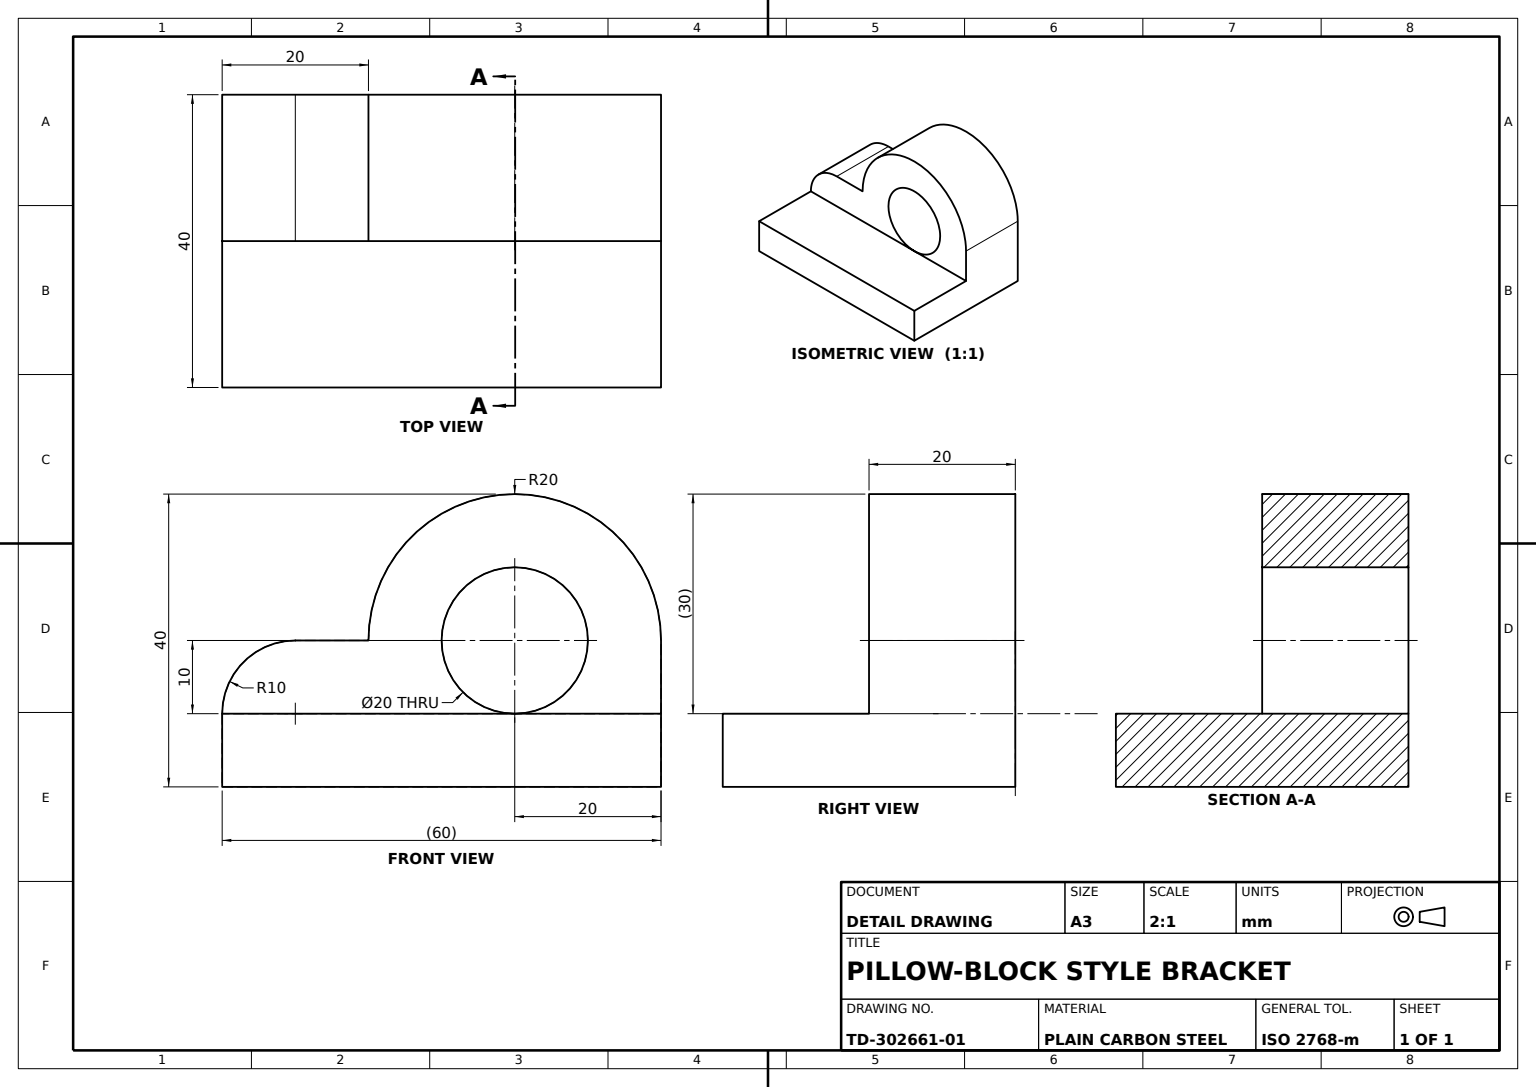
SolidWorks part; units mm, degrees
material "Plain Carbon Steel"
ref_plane "Front Plane" through (0, 0, 0) normal (0, 0, 1) x (1, 0, 0)
ref_plane "Top Plane" through (0, 0, 0) normal (0, 1, 0) x (1, 0, 0)
ref_plane "Right Plane" through (0, 0, 0) normal (1, 0, 0) x (0, 0, -1)
sketch "Base Plate Sketch" plane through (0, 0, 0) normal (0, 1, 0) x (1, 0, 0)
  line L1 (-30, -20) -> (30, -20)
  line L2 (-30, -20) -> (-30, 20)
  line L3 (-30, 20) -> (30, 20)
  line L4 (30, -20) -> (30, 20)
  line L5 (-30, -20) -> (30, 20) construction
  line L6 (-30, 20) -> (30, -20) construction
  point P0 (0, 0)
  dimension "D1" = 60
  dimension "D2" = 40
extrude "Base Plate 60x40x10" add sketch "Base Plate Sketch" along normal mid plane 10
sketch "Upright Lug Sketch" plane through (0, 5, 0) normal (0, 1, 0) x (1, 0, 0)
  line L0 (30, -20) -> (30, 20) construction
  line L1 (-30, 20) -> (30, 20)
  line L2 (-30, 20) -> (-30, 0)
  line L3 (-30, 0) -> (30, 0)
  line L4 (30, 20) -> (30, 0)
extrude "Upright Lug" add sketch "Upright Lug Sketch" along normal blind 30
sketch "Cross Hole Sketch" plane through (0, 0, -20) normal (0, 0, -1) x (-1, 0, 0)
  line L0 (-30, 35) -> (-30, -5) construction
  line L1 (-30, -5) -> (30, -5) construction
  circle A0 centre (-10, 15) radius 10
  arc A1 (10, 15) -> (-30, 15) centre (-10, 15) ccw
  point P10 (-10, 15)
  dimension "D1" = 20
  dimension "D2" = 40
  dimension "D3" = 20
  dimension "D4" = 20
extrude "Cross Hole Cut" cut sketch "Cross Hole Sketch" against normal through all contours A0
sketch "Lug Profile Sketch" plane through (0, 0, -20) normal (0, 0, -1) x (-1, 0, 0)
  line L0 (-50, 15) -> (30, 15)
  line L1 (30, 35) -> (30, -5) construction
  line L2 (30, 35) -> (30, -5)
  line L3 (-30, 35) -> (-30, -5) construction
  line L4 (-30, 35) -> (-30, -5)
  line L5 (-30, 35) -> (30, 35) construction
  line L6 (-30, 35) -> (30, 35)
  circle A0 centre (-10, 15) radius 20
  point P6 (-10, 15)
  line M8 (30, -5) -> (30, 35)
  line M9 (30, 35) -> (-30, 35)
  line M10 (-30, 35) -> (-30, -5)
  dimension "D1" = 40
extrude "Lug Profile Cut" cut sketch "Lug Profile Sketch" against normal through all contours A0 L6 M10 | A0 L0 M8 M9
fillet "Lug Round R10" radius 10 1 edges at (-30, 15, -10)
